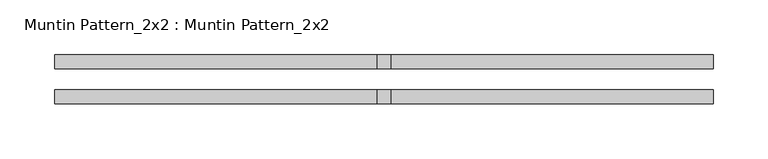
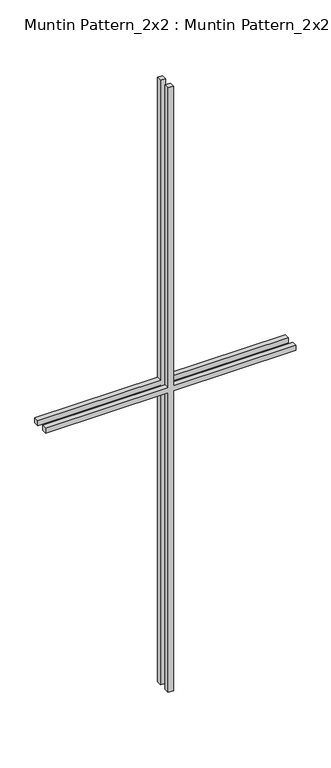
"""IFC4 building model written with IfcOpenShell, lengths in millimetres: proxy geometry, Muntin Pattern_2x2 : Muntin Pattern_2x2."""

from ifc_helpers import new_model, si_unit, frame, origin, place, context, project, spatial, polyline, outline, extrude, source, transform, mapped, element, save


def muntin_pattern_2x2_muntin_pattern_2x2_111b6719(model_context):
    return source(origin(), model_context, "Body", "SweptSolid", [
        extrude(outline(polyline([(771.525, -6.35), (771.525, -300.0375), (758.825, -300.0375), (758.825, -6.35), (0.0, -6.35), (0.0, 6.35), (758.825, 6.35), (758.825, 300.0375), (771.525, 300.0375), (771.525, 6.35), (1530.35, 6.35), (1530.35, -6.35), (771.525, -6.35)])), frame((0.0, 9.525, 0.0), z_axis=(0.0, 1.0, 0.0), x_axis=(0.0, 0.0, 1.0)), (0.0, 0.0, 1.0), 12.7),
        extrude(outline(polyline([(771.525, -6.35), (771.525, -300.0375), (758.825, -300.0375), (758.825, -6.35), (0.0, -6.35), (0.0, 6.35), (758.825, 6.35), (758.825, 300.0375), (771.525, 300.0375), (771.525, 6.35), (1530.35, 6.35), (1530.35, -6.35), (771.525, -6.35)])), frame((0.0, -22.225, 0.0), z_axis=(0.0, 1.0, 0.0), x_axis=(0.0, 0.0, 1.0)), (0.0, 0.0, 1.0), 12.7),
    ])


if __name__ == "__main__":
    model = new_model("IFC4")
    model_context = context("Model", 3, world=origin())
    ifc_project = project(units=[si_unit("LENGTHUNIT", "METRE", prefix="MILLI")], contexts=[model_context])
    site = spatial("IfcSite", under=ifc_project)
    building = spatial("IfcBuilding", under=site)
    placement = place(None, origin())
    muntin_pattern_2x2_muntin_pattern_2x2_shape = muntin_pattern_2x2_muntin_pattern_2x2_111b6719(model_context)
    element("IfcBuildingElementProxy", 1, Name="Muntin Pattern_2x2 : Muntin Pattern_2x2", ObjectType="Muntin Pattern_2x2 : Muntin Pattern_2x2", at=placement, inside=building, context=model_context, shape_type="MappedRepresentation", body=[
        mapped(muntin_pattern_2x2_muntin_pattern_2x2_shape, transform((0.0, 0.0, 0.0), x_axis=(1.0, 0.0, 0.0), y_axis=(0.0, 1.0, 0.0), z_axis=(0.0, 0.0, 1.0))),
    ])
    save(model, "model.ifc")

# Revit data of these elements
# Type "Muntin Pattern_2x2 : Muntin Pattern_2x2"
#   Width [instance default] = 4' - 0"
#   Thickness = 0' - 0 1/2"
#   Height [instance default] = 4' - 0"
#   Distance = 0' - 0 3/4"
#   Interior Material [instance default] = none
#   Exterior Material [instance default] = none
#   Default Elevation = 0
# Element 1 (IfcBuildingElementProxy, "Muntin Pattern_2x2 : Muntin Pattern_2x2")
#   Width = 1' - 11 5/8"
#   Height = 5' - 0 1/4"
#   Interior Material = Wood - Stained
#   Exterior Material = Clad - White
#   Materials on its faces: "Clad - White", "Wood - Stained"
# Materials
#   "Clad - White": class "Wood", colour RGB 242 242 238, transparency 0, Cost = 0
#   "Wood - Stained": class "Wood", colour RGB 224 178 126, transparency 0, Cost = 0
